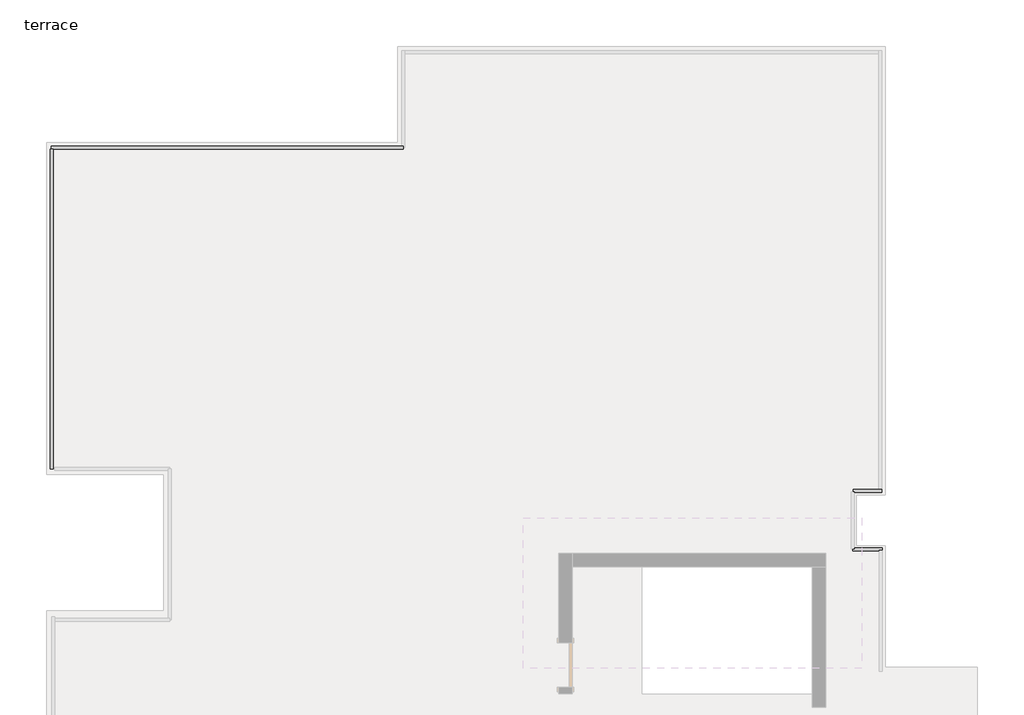
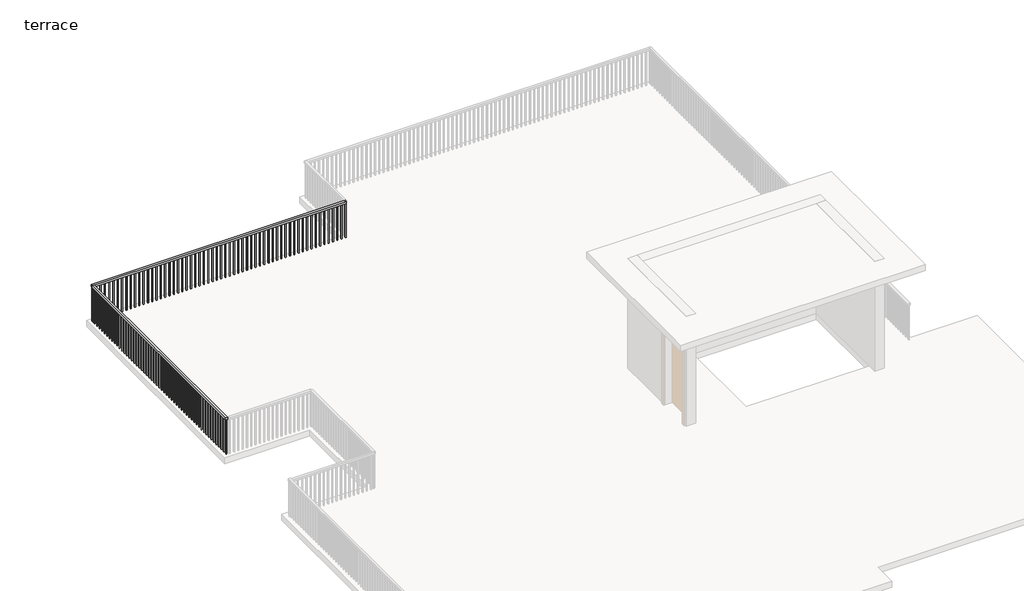
# One storey, part 5 of 7: 4 railings.
"""IFC4 building model written with IfcOpenShell, lengths in millimetres."""

from ifc_helpers import new_model, si_unit, frame, origin, place, context, project, spatial, polyline, outline, extrude, element, save

model = new_model("IFC4")

# Units and contexts
model_context = context("Model", 3, world=origin())
ifc_project = project(units=[si_unit("LENGTHUNIT", "METRE", prefix="MILLI")], contexts=[model_context])

# Site, building, storey
site = spatial("IfcSite", under=ifc_project)
building = spatial("IfcBuilding", under=site)
storey = spatial("IfcBuildingStorey", under=building, Name="terrace", Elevation=3810.0)

# Railings
placement = place(None, origin())
element("IfcRailing", 1, ObjectType="Handrail - Rectangular", at=placement, inside=storey, context=model_context, shape_type="SweptSolid", body=[
    extrude(outline(polyline([(-14404.2890129, 10982.627622), (-14404.2890129, 11033.427622), (-8409.8890129, 11033.427622), (-8409.8890129, 10982.627622), (-14404.2890129, 10982.627622)])), frame((0.0, 0.0, 4673.6), z_axis=(0.0, 0.0, 1.0), x_axis=(1.0, 0.0, 0.0)), (0.0, 0.0, 1.0), 50.8),
    extrude(outline(polyline([(-8521.0140129, 10998.502622), (-8521.0140129, 11017.552622), (-8501.9640129, 11017.552622), (-8501.9640129, 10998.502622), (-8521.0140129, 10998.502622)])), frame((0.0, 0.0, 3810.0), z_axis=(0.0, 0.0, 1.0), x_axis=(1.0, 0.0, 0.0)), (0.0, 0.0, 1.0), 863.6),
    extrude(outline(polyline([(-8622.6140129, 10998.502622), (-8622.6140129, 11017.552622), (-8603.5640129, 11017.552622), (-8603.5640129, 10998.502622), (-8622.6140129, 10998.502622)])), frame((0.0, 0.0, 3810.0), z_axis=(0.0, 0.0, 1.0), x_axis=(1.0, 0.0, 0.0)), (0.0, 0.0, 1.0), 863.6),
    extrude(outline(polyline([(-8724.2140129, 10998.502622), (-8724.2140129, 11017.552622), (-8705.1640129, 11017.552622), (-8705.1640129, 10998.502622), (-8724.2140129, 10998.502622)])), frame((0.0, 0.0, 3810.0), z_axis=(0.0, 0.0, 1.0), x_axis=(1.0, 0.0, 0.0)), (0.0, 0.0, 1.0), 863.6),
    extrude(outline(polyline([(-8825.8140129, 10998.502622), (-8825.8140129, 11017.552622), (-8806.7640129, 11017.552622), (-8806.7640129, 10998.502622), (-8825.8140129, 10998.502622)])), frame((0.0, 0.0, 3810.0), z_axis=(0.0, 0.0, 1.0), x_axis=(1.0, 0.0, 0.0)), (0.0, 0.0, 1.0), 863.6),
    extrude(outline(polyline([(-8927.4140129, 10998.502622), (-8927.4140129, 11017.552622), (-8908.3640129, 11017.552622), (-8908.3640129, 10998.502622), (-8927.4140129, 10998.502622)])), frame((0.0, 0.0, 3810.0), z_axis=(0.0, 0.0, 1.0), x_axis=(1.0, 0.0, 0.0)), (0.0, 0.0, 1.0), 863.6),
    extrude(outline(polyline([(-9029.0140129, 10998.502622), (-9029.0140129, 11017.552622), (-9009.9640129, 11017.552622), (-9009.9640129, 10998.502622), (-9029.0140129, 10998.502622)])), frame((0.0, 0.0, 3810.0), z_axis=(0.0, 0.0, 1.0), x_axis=(1.0, 0.0, 0.0)), (0.0, 0.0, 1.0), 863.6),
    extrude(outline(polyline([(-9130.6140129, 10998.502622), (-9130.6140129, 11017.552622), (-9111.5640129, 11017.552622), (-9111.5640129, 10998.502622), (-9130.6140129, 10998.502622)])), frame((0.0, 0.0, 3810.0), z_axis=(0.0, 0.0, 1.0), x_axis=(1.0, 0.0, 0.0)), (0.0, 0.0, 1.0), 863.6),
    extrude(outline(polyline([(-9232.2140129, 10998.502622), (-9232.2140129, 11017.552622), (-9213.1640129, 11017.552622), (-9213.1640129, 10998.502622), (-9232.2140129, 10998.502622)])), frame((0.0, 0.0, 3810.0), z_axis=(0.0, 0.0, 1.0), x_axis=(1.0, 0.0, 0.0)), (0.0, 0.0, 1.0), 863.6),
    extrude(outline(polyline([(-9333.8140129, 10998.502622), (-9333.8140129, 11017.552622), (-9314.7640129, 11017.552622), (-9314.7640129, 10998.502622), (-9333.8140129, 10998.502622)])), frame((0.0, 0.0, 3810.0), z_axis=(0.0, 0.0, 1.0), x_axis=(1.0, 0.0, 0.0)), (0.0, 0.0, 1.0), 863.6),
    extrude(outline(polyline([(-9435.4140129, 10998.502622), (-9435.4140129, 11017.552622), (-9416.3640129, 11017.552622), (-9416.3640129, 10998.502622), (-9435.4140129, 10998.502622)])), frame((0.0, 0.0, 3810.0), z_axis=(0.0, 0.0, 1.0), x_axis=(1.0, 0.0, 0.0)), (0.0, 0.0, 1.0), 863.6),
    extrude(outline(polyline([(-9537.0140129, 10998.502622), (-9537.0140129, 11017.552622), (-9517.9640129, 11017.552622), (-9517.9640129, 10998.502622), (-9537.0140129, 10998.502622)])), frame((0.0, 0.0, 3810.0), z_axis=(0.0, 0.0, 1.0), x_axis=(1.0, 0.0, 0.0)), (0.0, 0.0, 1.0), 863.6),
    extrude(outline(polyline([(-9638.6140129, 10998.502622), (-9638.6140129, 11017.552622), (-9619.5640129, 11017.552622), (-9619.5640129, 10998.502622), (-9638.6140129, 10998.502622)])), frame((0.0, 0.0, 3810.0), z_axis=(0.0, 0.0, 1.0), x_axis=(1.0, 0.0, 0.0)), (0.0, 0.0, 1.0), 863.6),
    extrude(outline(polyline([(-9740.2140129, 10998.502622), (-9740.2140129, 11017.552622), (-9721.1640129, 11017.552622), (-9721.1640129, 10998.502622), (-9740.2140129, 10998.502622)])), frame((0.0, 0.0, 3810.0), z_axis=(0.0, 0.0, 1.0), x_axis=(1.0, 0.0, 0.0)), (0.0, 0.0, 1.0), 863.6),
    extrude(outline(polyline([(-9841.8140129, 10998.502622), (-9841.8140129, 11017.552622), (-9822.7640129, 11017.552622), (-9822.7640129, 10998.502622), (-9841.8140129, 10998.502622)])), frame((0.0, 0.0, 3810.0), z_axis=(0.0, 0.0, 1.0), x_axis=(1.0, 0.0, 0.0)), (0.0, 0.0, 1.0), 863.6),
    extrude(outline(polyline([(-9943.4140129, 10998.502622), (-9943.4140129, 11017.552622), (-9924.3640129, 11017.552622), (-9924.3640129, 10998.502622), (-9943.4140129, 10998.502622)])), frame((0.0, 0.0, 3810.0), z_axis=(0.0, 0.0, 1.0), x_axis=(1.0, 0.0, 0.0)), (0.0, 0.0, 1.0), 863.6),
    extrude(outline(polyline([(-10045.0140129, 10998.502622), (-10045.0140129, 11017.552622), (-10025.9640129, 11017.552622), (-10025.9640129, 10998.502622), (-10045.0140129, 10998.502622)])), frame((0.0, 0.0, 3810.0), z_axis=(0.0, 0.0, 1.0), x_axis=(1.0, 0.0, 0.0)), (0.0, 0.0, 1.0), 863.6),
    extrude(outline(polyline([(-10146.6140129, 10998.502622), (-10146.6140129, 11017.552622), (-10127.5640129, 11017.552622), (-10127.5640129, 10998.502622), (-10146.6140129, 10998.502622)])), frame((0.0, 0.0, 3810.0), z_axis=(0.0, 0.0, 1.0), x_axis=(1.0, 0.0, 0.0)), (0.0, 0.0, 1.0), 863.6),
    extrude(outline(polyline([(-10248.2140129, 10998.502622), (-10248.2140129, 11017.552622), (-10229.1640129, 11017.552622), (-10229.1640129, 10998.502622), (-10248.2140129, 10998.502622)])), frame((0.0, 0.0, 3810.0), z_axis=(0.0, 0.0, 1.0), x_axis=(1.0, 0.0, 0.0)), (0.0, 0.0, 1.0), 863.6),
    extrude(outline(polyline([(-10349.8140129, 10998.502622), (-10349.8140129, 11017.552622), (-10330.7640129, 11017.552622), (-10330.7640129, 10998.502622), (-10349.8140129, 10998.502622)])), frame((0.0, 0.0, 3810.0), z_axis=(0.0, 0.0, 1.0), x_axis=(1.0, 0.0, 0.0)), (0.0, 0.0, 1.0), 863.6),
    extrude(outline(polyline([(-10451.4140129, 10998.502622), (-10451.4140129, 11017.552622), (-10432.3640129, 11017.552622), (-10432.3640129, 10998.502622), (-10451.4140129, 10998.502622)])), frame((0.0, 0.0, 3810.0), z_axis=(0.0, 0.0, 1.0), x_axis=(1.0, 0.0, 0.0)), (0.0, 0.0, 1.0), 863.6),
    extrude(outline(polyline([(-10553.0140129, 10998.502622), (-10553.0140129, 11017.552622), (-10533.9640129, 11017.552622), (-10533.9640129, 10998.502622), (-10553.0140129, 10998.502622)])), frame((0.0, 0.0, 3810.0), z_axis=(0.0, 0.0, 1.0), x_axis=(1.0, 0.0, 0.0)), (0.0, 0.0, 1.0), 863.6),
    extrude(outline(polyline([(-10654.6140129, 10998.502622), (-10654.6140129, 11017.552622), (-10635.5640129, 11017.552622), (-10635.5640129, 10998.502622), (-10654.6140129, 10998.502622)])), frame((0.0, 0.0, 3810.0), z_axis=(0.0, 0.0, 1.0), x_axis=(1.0, 0.0, 0.0)), (0.0, 0.0, 1.0), 863.6),
    extrude(outline(polyline([(-10756.2140129, 10998.502622), (-10756.2140129, 11017.552622), (-10737.1640129, 11017.552622), (-10737.1640129, 10998.502622), (-10756.2140129, 10998.502622)])), frame((0.0, 0.0, 3810.0), z_axis=(0.0, 0.0, 1.0), x_axis=(1.0, 0.0, 0.0)), (0.0, 0.0, 1.0), 863.6),
    extrude(outline(polyline([(-10857.8140129, 10998.502622), (-10857.8140129, 11017.552622), (-10838.7640129, 11017.552622), (-10838.7640129, 10998.502622), (-10857.8140129, 10998.502622)])), frame((0.0, 0.0, 3810.0), z_axis=(0.0, 0.0, 1.0), x_axis=(1.0, 0.0, 0.0)), (0.0, 0.0, 1.0), 863.6),
    extrude(outline(polyline([(-10959.4140129, 10998.502622), (-10959.4140129, 11017.552622), (-10940.3640129, 11017.552622), (-10940.3640129, 10998.502622), (-10959.4140129, 10998.502622)])), frame((0.0, 0.0, 3810.0), z_axis=(0.0, 0.0, 1.0), x_axis=(1.0, 0.0, 0.0)), (0.0, 0.0, 1.0), 863.6),
    extrude(outline(polyline([(-11061.0140129, 10998.502622), (-11061.0140129, 11017.552622), (-11041.9640129, 11017.552622), (-11041.9640129, 10998.502622), (-11061.0140129, 10998.502622)])), frame((0.0, 0.0, 3810.0), z_axis=(0.0, 0.0, 1.0), x_axis=(1.0, 0.0, 0.0)), (0.0, 0.0, 1.0), 863.6),
    extrude(outline(polyline([(-11162.6140129, 10998.502622), (-11162.6140129, 11017.552622), (-11143.5640129, 11017.552622), (-11143.5640129, 10998.502622), (-11162.6140129, 10998.502622)])), frame((0.0, 0.0, 3810.0), z_axis=(0.0, 0.0, 1.0), x_axis=(1.0, 0.0, 0.0)), (0.0, 0.0, 1.0), 863.6),
    extrude(outline(polyline([(-11264.2140129, 10998.502622), (-11264.2140129, 11017.552622), (-11245.1640129, 11017.552622), (-11245.1640129, 10998.502622), (-11264.2140129, 10998.502622)])), frame((0.0, 0.0, 3810.0), z_axis=(0.0, 0.0, 1.0), x_axis=(1.0, 0.0, 0.0)), (0.0, 0.0, 1.0), 863.6),
    extrude(outline(polyline([(-11365.8140129, 10998.502622), (-11365.8140129, 11017.552622), (-11346.7640129, 11017.552622), (-11346.7640129, 10998.502622), (-11365.8140129, 10998.502622)])), frame((0.0, 0.0, 3810.0), z_axis=(0.0, 0.0, 1.0), x_axis=(1.0, 0.0, 0.0)), (0.0, 0.0, 1.0), 863.6),
    extrude(outline(polyline([(-11467.4140129, 10998.502622), (-11467.4140129, 11017.552622), (-11448.3640129, 11017.552622), (-11448.3640129, 10998.502622), (-11467.4140129, 10998.502622)])), frame((0.0, 0.0, 3810.0), z_axis=(0.0, 0.0, 1.0), x_axis=(1.0, 0.0, 0.0)), (0.0, 0.0, 1.0), 863.6),
    extrude(outline(polyline([(-11569.0140129, 10998.502622), (-11569.0140129, 11017.552622), (-11549.9640129, 11017.552622), (-11549.9640129, 10998.502622), (-11569.0140129, 10998.502622)])), frame((0.0, 0.0, 3810.0), z_axis=(0.0, 0.0, 1.0), x_axis=(1.0, 0.0, 0.0)), (0.0, 0.0, 1.0), 863.6),
    extrude(outline(polyline([(-11670.6140129, 10998.502622), (-11670.6140129, 11017.552622), (-11651.5640129, 11017.552622), (-11651.5640129, 10998.502622), (-11670.6140129, 10998.502622)])), frame((0.0, 0.0, 3810.0), z_axis=(0.0, 0.0, 1.0), x_axis=(1.0, 0.0, 0.0)), (0.0, 0.0, 1.0), 863.6),
    extrude(outline(polyline([(-11772.2140129, 10998.502622), (-11772.2140129, 11017.552622), (-11753.1640129, 11017.552622), (-11753.1640129, 10998.502622), (-11772.2140129, 10998.502622)])), frame((0.0, 0.0, 3810.0), z_axis=(0.0, 0.0, 1.0), x_axis=(1.0, 0.0, 0.0)), (0.0, 0.0, 1.0), 863.6),
    extrude(outline(polyline([(-11873.8140129, 10998.502622), (-11873.8140129, 11017.552622), (-11854.7640129, 11017.552622), (-11854.7640129, 10998.502622), (-11873.8140129, 10998.502622)])), frame((0.0, 0.0, 3810.0), z_axis=(0.0, 0.0, 1.0), x_axis=(1.0, 0.0, 0.0)), (0.0, 0.0, 1.0), 863.6),
    extrude(outline(polyline([(-11975.4140129, 10998.502622), (-11975.4140129, 11017.552622), (-11956.3640129, 11017.552622), (-11956.3640129, 10998.502622), (-11975.4140129, 10998.502622)])), frame((0.0, 0.0, 3810.0), z_axis=(0.0, 0.0, 1.0), x_axis=(1.0, 0.0, 0.0)), (0.0, 0.0, 1.0), 863.6),
    extrude(outline(polyline([(-12077.0140129, 10998.502622), (-12077.0140129, 11017.552622), (-12057.9640129, 11017.552622), (-12057.9640129, 10998.502622), (-12077.0140129, 10998.502622)])), frame((0.0, 0.0, 3810.0), z_axis=(0.0, 0.0, 1.0), x_axis=(1.0, 0.0, 0.0)), (0.0, 0.0, 1.0), 863.6),
    extrude(outline(polyline([(-12178.6140129, 10998.502622), (-12178.6140129, 11017.552622), (-12159.5640129, 11017.552622), (-12159.5640129, 10998.502622), (-12178.6140129, 10998.502622)])), frame((0.0, 0.0, 3810.0), z_axis=(0.0, 0.0, 1.0), x_axis=(1.0, 0.0, 0.0)), (0.0, 0.0, 1.0), 863.6),
    extrude(outline(polyline([(-12280.2140129, 10998.502622), (-12280.2140129, 11017.552622), (-12261.1640129, 11017.552622), (-12261.1640129, 10998.502622), (-12280.2140129, 10998.502622)])), frame((0.0, 0.0, 3810.0), z_axis=(0.0, 0.0, 1.0), x_axis=(1.0, 0.0, 0.0)), (0.0, 0.0, 1.0), 863.6),
    extrude(outline(polyline([(-12381.8140129, 10998.502622), (-12381.8140129, 11017.552622), (-12362.7640129, 11017.552622), (-12362.7640129, 10998.502622), (-12381.8140129, 10998.502622)])), frame((0.0, 0.0, 3810.0), z_axis=(0.0, 0.0, 1.0), x_axis=(1.0, 0.0, 0.0)), (0.0, 0.0, 1.0), 863.6),
    extrude(outline(polyline([(-12483.4140129, 10998.502622), (-12483.4140129, 11017.552622), (-12464.3640129, 11017.552622), (-12464.3640129, 10998.502622), (-12483.4140129, 10998.502622)])), frame((0.0, 0.0, 3810.0), z_axis=(0.0, 0.0, 1.0), x_axis=(1.0, 0.0, 0.0)), (0.0, 0.0, 1.0), 863.6),
    extrude(outline(polyline([(-12585.0140129, 10998.502622), (-12585.0140129, 11017.552622), (-12565.9640129, 11017.552622), (-12565.9640129, 10998.502622), (-12585.0140129, 10998.502622)])), frame((0.0, 0.0, 3810.0), z_axis=(0.0, 0.0, 1.0), x_axis=(1.0, 0.0, 0.0)), (0.0, 0.0, 1.0), 863.6),
    extrude(outline(polyline([(-12686.6140129, 10998.502622), (-12686.6140129, 11017.552622), (-12667.5640129, 11017.552622), (-12667.5640129, 10998.502622), (-12686.6140129, 10998.502622)])), frame((0.0, 0.0, 3810.0), z_axis=(0.0, 0.0, 1.0), x_axis=(1.0, 0.0, 0.0)), (0.0, 0.0, 1.0), 863.6),
    extrude(outline(polyline([(-12788.2140129, 10998.502622), (-12788.2140129, 11017.552622), (-12769.1640129, 11017.552622), (-12769.1640129, 10998.502622), (-12788.2140129, 10998.502622)])), frame((0.0, 0.0, 3810.0), z_axis=(0.0, 0.0, 1.0), x_axis=(1.0, 0.0, 0.0)), (0.0, 0.0, 1.0), 863.6),
    extrude(outline(polyline([(-12889.8140129, 10998.502622), (-12889.8140129, 11017.552622), (-12870.7640129, 11017.552622), (-12870.7640129, 10998.502622), (-12889.8140129, 10998.502622)])), frame((0.0, 0.0, 3810.0), z_axis=(0.0, 0.0, 1.0), x_axis=(1.0, 0.0, 0.0)), (0.0, 0.0, 1.0), 863.6),
    extrude(outline(polyline([(-12991.4140129, 10998.502622), (-12991.4140129, 11017.552622), (-12972.3640129, 11017.552622), (-12972.3640129, 10998.502622), (-12991.4140129, 10998.502622)])), frame((0.0, 0.0, 3810.0), z_axis=(0.0, 0.0, 1.0), x_axis=(1.0, 0.0, 0.0)), (0.0, 0.0, 1.0), 863.6),
    extrude(outline(polyline([(-13093.0140129, 10998.502622), (-13093.0140129, 11017.552622), (-13073.9640129, 11017.552622), (-13073.9640129, 10998.502622), (-13093.0140129, 10998.502622)])), frame((0.0, 0.0, 3810.0), z_axis=(0.0, 0.0, 1.0), x_axis=(1.0, 0.0, 0.0)), (0.0, 0.0, 1.0), 863.6),
    extrude(outline(polyline([(-13194.6140129, 10998.502622), (-13194.6140129, 11017.552622), (-13175.5640129, 11017.552622), (-13175.5640129, 10998.502622), (-13194.6140129, 10998.502622)])), frame((0.0, 0.0, 3810.0), z_axis=(0.0, 0.0, 1.0), x_axis=(1.0, 0.0, 0.0)), (0.0, 0.0, 1.0), 863.6),
    extrude(outline(polyline([(-13296.2140129, 10998.502622), (-13296.2140129, 11017.552622), (-13277.1640129, 11017.552622), (-13277.1640129, 10998.502622), (-13296.2140129, 10998.502622)])), frame((0.0, 0.0, 3810.0), z_axis=(0.0, 0.0, 1.0), x_axis=(1.0, 0.0, 0.0)), (0.0, 0.0, 1.0), 863.6),
    extrude(outline(polyline([(-13397.8140129, 10998.502622), (-13397.8140129, 11017.552622), (-13378.7640129, 11017.552622), (-13378.7640129, 10998.502622), (-13397.8140129, 10998.502622)])), frame((0.0, 0.0, 3810.0), z_axis=(0.0, 0.0, 1.0), x_axis=(1.0, 0.0, 0.0)), (0.0, 0.0, 1.0), 863.6),
    extrude(outline(polyline([(-13499.4140129, 10998.502622), (-13499.4140129, 11017.552622), (-13480.3640129, 11017.552622), (-13480.3640129, 10998.502622), (-13499.4140129, 10998.502622)])), frame((0.0, 0.0, 3810.0), z_axis=(0.0, 0.0, 1.0), x_axis=(1.0, 0.0, 0.0)), (0.0, 0.0, 1.0), 863.6),
    extrude(outline(polyline([(-13601.0140129, 10998.502622), (-13601.0140129, 11017.552622), (-13581.9640129, 11017.552622), (-13581.9640129, 10998.502622), (-13601.0140129, 10998.502622)])), frame((0.0, 0.0, 3810.0), z_axis=(0.0, 0.0, 1.0), x_axis=(1.0, 0.0, 0.0)), (0.0, 0.0, 1.0), 863.6),
    extrude(outline(polyline([(-13702.6140129, 10998.502622), (-13702.6140129, 11017.552622), (-13683.5640129, 11017.552622), (-13683.5640129, 10998.502622), (-13702.6140129, 10998.502622)])), frame((0.0, 0.0, 3810.0), z_axis=(0.0, 0.0, 1.0), x_axis=(1.0, 0.0, 0.0)), (0.0, 0.0, 1.0), 863.6),
    extrude(outline(polyline([(-13804.2140129, 10998.502622), (-13804.2140129, 11017.552622), (-13785.1640129, 11017.552622), (-13785.1640129, 10998.502622), (-13804.2140129, 10998.502622)])), frame((0.0, 0.0, 3810.0), z_axis=(0.0, 0.0, 1.0), x_axis=(1.0, 0.0, 0.0)), (0.0, 0.0, 1.0), 863.6),
    extrude(outline(polyline([(-13905.8140129, 10998.502622), (-13905.8140129, 11017.552622), (-13886.7640129, 11017.552622), (-13886.7640129, 10998.502622), (-13905.8140129, 10998.502622)])), frame((0.0, 0.0, 3810.0), z_axis=(0.0, 0.0, 1.0), x_axis=(1.0, 0.0, 0.0)), (0.0, 0.0, 1.0), 863.6),
    extrude(outline(polyline([(-14007.4140129, 10998.502622), (-14007.4140129, 11017.552622), (-13988.3640129, 11017.552622), (-13988.3640129, 10998.502622), (-14007.4140129, 10998.502622)])), frame((0.0, 0.0, 3810.0), z_axis=(0.0, 0.0, 1.0), x_axis=(1.0, 0.0, 0.0)), (0.0, 0.0, 1.0), 863.6),
    extrude(outline(polyline([(-14109.0140129, 10998.502622), (-14109.0140129, 11017.552622), (-14089.9640129, 11017.552622), (-14089.9640129, 10998.502622), (-14109.0140129, 10998.502622)])), frame((0.0, 0.0, 3810.0), z_axis=(0.0, 0.0, 1.0), x_axis=(1.0, 0.0, 0.0)), (0.0, 0.0, 1.0), 863.6),
    extrude(outline(polyline([(-14210.6140129, 10998.502622), (-14210.6140129, 11017.552622), (-14191.5640129, 11017.552622), (-14191.5640129, 10998.502622), (-14210.6140129, 10998.502622)])), frame((0.0, 0.0, 3810.0), z_axis=(0.0, 0.0, 1.0), x_axis=(1.0, 0.0, 0.0)), (0.0, 0.0, 1.0), 863.6),
    extrude(outline(polyline([(-14312.2140129, 10998.502622), (-14312.2140129, 11017.552622), (-14293.1640129, 11017.552622), (-14293.1640129, 10998.502622), (-14312.2140129, 10998.502622)])), frame((0.0, 0.0, 3810.0), z_axis=(0.0, 0.0, 1.0), x_axis=(1.0, 0.0, 0.0)), (0.0, 0.0, 1.0), 863.6),
    extrude(outline(polyline([(-8428.9390129, 10998.502622), (-8428.9390129, 11017.552622), (-8409.8890129, 11017.552622), (-8409.8890129, 10998.502622), (-8428.9390129, 10998.502622)])), frame((0.0, 0.0, 3810.0), z_axis=(0.0, 0.0, 1.0), x_axis=(1.0, 0.0, 0.0)), (0.0, 0.0, 1.0), 863.6),
    extrude(outline(polyline([(-14404.2890129, 10998.502622), (-14404.2890129, 11017.552622), (-14385.2390129, 11017.552622), (-14385.2390129, 10998.502622), (-14404.2890129, 10998.502622)])), frame((0.0, 0.0, 3810.0), z_axis=(0.0, 0.0, 1.0), x_axis=(1.0, 0.0, 0.0)), (0.0, 0.0, 1.0), 863.6),
])
element("IfcRailing", 2, ObjectType="Handrail - Rectangular", at=placement, inside=storey, context=model_context, shape_type="SweptSolid", body=[
    extrude(outline(polyline([(-256.4890129, 5178.727622), (-256.4890129, 5127.927622), (-739.0890129, 5127.927622), (-739.0890129, 5178.727622), (-256.4890129, 5178.727622)])), frame((0.0, 0.0, 4673.6), z_axis=(0.0, 0.0, 1.0), x_axis=(1.0, 0.0, 0.0)), (0.0, 0.0, 1.0), 50.8),
    extrude(outline(polyline([(-653.3640129, 5162.852622), (-653.3640129, 5143.802622), (-672.4140129, 5143.802622), (-672.4140129, 5162.852622), (-653.3640129, 5162.852622)])), frame((0.0, 0.0, 3810.0), z_axis=(0.0, 0.0, 1.0), x_axis=(1.0, 0.0, 0.0)), (0.0, 0.0, 1.0), 863.6),
    extrude(outline(polyline([(-551.7640129, 5162.852622), (-551.7640129, 5143.802622), (-570.8140129, 5143.802622), (-570.8140129, 5162.852622), (-551.7640129, 5162.852622)])), frame((0.0, 0.0, 3810.0), z_axis=(0.0, 0.0, 1.0), x_axis=(1.0, 0.0, 0.0)), (0.0, 0.0, 1.0), 863.6),
    extrude(outline(polyline([(-450.1640129, 5162.852622), (-450.1640129, 5143.802622), (-469.2140129, 5143.802622), (-469.2140129, 5162.852622), (-450.1640129, 5162.852622)])), frame((0.0, 0.0, 3810.0), z_axis=(0.0, 0.0, 1.0), x_axis=(1.0, 0.0, 0.0)), (0.0, 0.0, 1.0), 863.6),
    extrude(outline(polyline([(-348.5640129, 5162.852622), (-348.5640129, 5143.802622), (-367.6140129, 5143.802622), (-367.6140129, 5162.852622), (-348.5640129, 5162.852622)])), frame((0.0, 0.0, 3810.0), z_axis=(0.0, 0.0, 1.0), x_axis=(1.0, 0.0, 0.0)), (0.0, 0.0, 1.0), 863.6),
    extrude(outline(polyline([(-720.0390129, 5162.852622), (-720.0390129, 5143.802622), (-739.0890129, 5143.802622), (-739.0890129, 5162.852622), (-720.0390129, 5162.852622)])), frame((0.0, 0.0, 3810.0), z_axis=(0.0, 0.0, 1.0), x_axis=(1.0, 0.0, 0.0)), (0.0, 0.0, 1.0), 863.6),
    extrude(outline(polyline([(-256.4890129, 5162.852622), (-256.4890129, 5143.802622), (-275.5390129, 5143.802622), (-275.5390129, 5162.852622), (-256.4890129, 5162.852622)])), frame((0.0, 0.0, 3810.0), z_axis=(0.0, 0.0, 1.0), x_axis=(1.0, 0.0, 0.0)), (0.0, 0.0, 1.0), 863.6),
])
element("IfcRailing", 3, ObjectType="Handrail - Rectangular", at=placement, inside=storey, context=model_context, shape_type="SweptSolid", body=[
    extrude(outline(polyline([(-751.7890129, 4130.977622), (-751.7890129, 4181.777622), (-243.7890129, 4181.777622), (-243.7890129, 4130.977622), (-751.7890129, 4130.977622)])), frame((0.0, 0.0, 4673.6), z_axis=(0.0, 0.0, 1.0), x_axis=(1.0, 0.0, 0.0)), (0.0, 0.0, 1.0), 50.8),
    extrude(outline(polyline([(-354.9140129, 4146.852622), (-354.9140129, 4165.902622), (-335.8640129, 4165.902622), (-335.8640129, 4146.852622), (-354.9140129, 4146.852622)])), frame((0.0, 0.0, 3810.0), z_axis=(0.0, 0.0, 1.0), x_axis=(1.0, 0.0, 0.0)), (0.0, 0.0, 1.0), 863.6),
    extrude(outline(polyline([(-456.5140129, 4146.852622), (-456.5140129, 4165.902622), (-437.4640129, 4165.902622), (-437.4640129, 4146.852622), (-456.5140129, 4146.852622)])), frame((0.0, 0.0, 3810.0), z_axis=(0.0, 0.0, 1.0), x_axis=(1.0, 0.0, 0.0)), (0.0, 0.0, 1.0), 863.6),
    extrude(outline(polyline([(-558.1140129, 4146.852622), (-558.1140129, 4165.902622), (-539.0640129, 4165.902622), (-539.0640129, 4146.852622), (-558.1140129, 4146.852622)])), frame((0.0, 0.0, 3810.0), z_axis=(0.0, 0.0, 1.0), x_axis=(1.0, 0.0, 0.0)), (0.0, 0.0, 1.0), 863.6),
    extrude(outline(polyline([(-659.7140129, 4146.852622), (-659.7140129, 4165.902622), (-640.6640129, 4165.902622), (-640.6640129, 4146.852622), (-659.7140129, 4146.852622)])), frame((0.0, 0.0, 3810.0), z_axis=(0.0, 0.0, 1.0), x_axis=(1.0, 0.0, 0.0)), (0.0, 0.0, 1.0), 863.6),
    extrude(outline(polyline([(-262.8390129, 4146.852622), (-262.8390129, 4165.902622), (-243.7890129, 4165.902622), (-243.7890129, 4146.852622), (-262.8390129, 4146.852622)])), frame((0.0, 0.0, 3810.0), z_axis=(0.0, 0.0, 1.0), x_axis=(1.0, 0.0, 0.0)), (0.0, 0.0, 1.0), 863.6),
    extrude(outline(polyline([(-751.7890129, 4146.852622), (-751.7890129, 4165.902622), (-732.7390129, 4165.902622), (-732.7390129, 4146.852622), (-751.7890129, 4146.852622)])), frame((0.0, 0.0, 3810.0), z_axis=(0.0, 0.0, 1.0), x_axis=(1.0, 0.0, 0.0)), (0.0, 0.0, 1.0), 863.6),
])
element("IfcRailing", 4, ObjectType="Handrail - Rectangular", at=placement, inside=storey, context=model_context, shape_type="SweptSolid", body=[
    extrude(outline(polyline([(-14366.1890129, 5527.977622), (-14416.9890129, 5527.977622), (-14416.9890129, 10982.627622), (-14366.1890129, 10982.627622), (-14366.1890129, 5527.977622)])), frame((0.0, 0.0, 4673.6), z_axis=(0.0, 0.0, 1.0), x_axis=(1.0, 0.0, 0.0)), (0.0, 0.0, 1.0), 50.8),
    extrude(outline(polyline([(-14382.0640129, 10903.252622), (-14401.1140129, 10903.252622), (-14401.1140129, 10922.302622), (-14382.0640129, 10922.302622), (-14382.0640129, 10903.252622)])), frame((0.0, 0.0, 3810.0), z_axis=(0.0, 0.0, 1.0), x_axis=(1.0, 0.0, 0.0)), (0.0, 0.0, 1.0), 863.6),
    extrude(outline(polyline([(-14382.0640129, 10801.652622), (-14401.1140129, 10801.652622), (-14401.1140129, 10820.702622), (-14382.0640129, 10820.702622), (-14382.0640129, 10801.652622)])), frame((0.0, 0.0, 3810.0), z_axis=(0.0, 0.0, 1.0), x_axis=(1.0, 0.0, 0.0)), (0.0, 0.0, 1.0), 863.6),
    extrude(outline(polyline([(-14382.0640129, 10700.052622), (-14401.1140129, 10700.052622), (-14401.1140129, 10719.102622), (-14382.0640129, 10719.102622), (-14382.0640129, 10700.052622)])), frame((0.0, 0.0, 3810.0), z_axis=(0.0, 0.0, 1.0), x_axis=(1.0, 0.0, 0.0)), (0.0, 0.0, 1.0), 863.6),
    extrude(outline(polyline([(-14382.0640129, 10598.452622), (-14401.1140129, 10598.452622), (-14401.1140129, 10617.502622), (-14382.0640129, 10617.502622), (-14382.0640129, 10598.452622)])), frame((0.0, 0.0, 3810.0), z_axis=(0.0, 0.0, 1.0), x_axis=(1.0, 0.0, 0.0)), (0.0, 0.0, 1.0), 863.6),
    extrude(outline(polyline([(-14382.0640129, 10496.852622), (-14401.1140129, 10496.852622), (-14401.1140129, 10515.902622), (-14382.0640129, 10515.902622), (-14382.0640129, 10496.852622)])), frame((0.0, 0.0, 3810.0), z_axis=(0.0, 0.0, 1.0), x_axis=(1.0, 0.0, 0.0)), (0.0, 0.0, 1.0), 863.6),
    extrude(outline(polyline([(-14382.0640129, 10395.252622), (-14401.1140129, 10395.252622), (-14401.1140129, 10414.302622), (-14382.0640129, 10414.302622), (-14382.0640129, 10395.252622)])), frame((0.0, 0.0, 3810.0), z_axis=(0.0, 0.0, 1.0), x_axis=(1.0, 0.0, 0.0)), (0.0, 0.0, 1.0), 863.6),
    extrude(outline(polyline([(-14382.0640129, 10293.652622), (-14401.1140129, 10293.652622), (-14401.1140129, 10312.702622), (-14382.0640129, 10312.702622), (-14382.0640129, 10293.652622)])), frame((0.0, 0.0, 3810.0), z_axis=(0.0, 0.0, 1.0), x_axis=(1.0, 0.0, 0.0)), (0.0, 0.0, 1.0), 863.6),
    extrude(outline(polyline([(-14382.0640129, 10192.052622), (-14401.1140129, 10192.052622), (-14401.1140129, 10211.102622), (-14382.0640129, 10211.102622), (-14382.0640129, 10192.052622)])), frame((0.0, 0.0, 3810.0), z_axis=(0.0, 0.0, 1.0), x_axis=(1.0, 0.0, 0.0)), (0.0, 0.0, 1.0), 863.6),
    extrude(outline(polyline([(-14382.0640129, 10090.452622), (-14401.1140129, 10090.452622), (-14401.1140129, 10109.502622), (-14382.0640129, 10109.502622), (-14382.0640129, 10090.452622)])), frame((0.0, 0.0, 3810.0), z_axis=(0.0, 0.0, 1.0), x_axis=(1.0, 0.0, 0.0)), (0.0, 0.0, 1.0), 863.6),
    extrude(outline(polyline([(-14382.0640129, 9988.852622), (-14401.1140129, 9988.852622), (-14401.1140129, 10007.902622), (-14382.0640129, 10007.902622), (-14382.0640129, 9988.852622)])), frame((0.0, 0.0, 3810.0), z_axis=(0.0, 0.0, 1.0), x_axis=(1.0, 0.0, 0.0)), (0.0, 0.0, 1.0), 863.6),
    extrude(outline(polyline([(-14382.0640129, 9887.252622), (-14401.1140129, 9887.252622), (-14401.1140129, 9906.302622), (-14382.0640129, 9906.302622), (-14382.0640129, 9887.252622)])), frame((0.0, 0.0, 3810.0), z_axis=(0.0, 0.0, 1.0), x_axis=(1.0, 0.0, 0.0)), (0.0, 0.0, 1.0), 863.6),
    extrude(outline(polyline([(-14382.0640129, 9785.652622), (-14401.1140129, 9785.652622), (-14401.1140129, 9804.702622), (-14382.0640129, 9804.702622), (-14382.0640129, 9785.652622)])), frame((0.0, 0.0, 3810.0), z_axis=(0.0, 0.0, 1.0), x_axis=(1.0, 0.0, 0.0)), (0.0, 0.0, 1.0), 863.6),
    extrude(outline(polyline([(-14382.0640129, 9684.052622), (-14401.1140129, 9684.052622), (-14401.1140129, 9703.102622), (-14382.0640129, 9703.102622), (-14382.0640129, 9684.052622)])), frame((0.0, 0.0, 3810.0), z_axis=(0.0, 0.0, 1.0), x_axis=(1.0, 0.0, 0.0)), (0.0, 0.0, 1.0), 863.6),
    extrude(outline(polyline([(-14382.0640129, 9582.452622), (-14401.1140129, 9582.452622), (-14401.1140129, 9601.502622), (-14382.0640129, 9601.502622), (-14382.0640129, 9582.452622)])), frame((0.0, 0.0, 3810.0), z_axis=(0.0, 0.0, 1.0), x_axis=(1.0, 0.0, 0.0)), (0.0, 0.0, 1.0), 863.6),
    extrude(outline(polyline([(-14382.0640129, 9480.852622), (-14401.1140129, 9480.852622), (-14401.1140129, 9499.902622), (-14382.0640129, 9499.902622), (-14382.0640129, 9480.852622)])), frame((0.0, 0.0, 3810.0), z_axis=(0.0, 0.0, 1.0), x_axis=(1.0, 0.0, 0.0)), (0.0, 0.0, 1.0), 863.6),
    extrude(outline(polyline([(-14382.0640129, 9379.252622), (-14401.1140129, 9379.252622), (-14401.1140129, 9398.302622), (-14382.0640129, 9398.302622), (-14382.0640129, 9379.252622)])), frame((0.0, 0.0, 3810.0), z_axis=(0.0, 0.0, 1.0), x_axis=(1.0, 0.0, 0.0)), (0.0, 0.0, 1.0), 863.6),
    extrude(outline(polyline([(-14382.0640129, 9277.652622), (-14401.1140129, 9277.652622), (-14401.1140129, 9296.702622), (-14382.0640129, 9296.702622), (-14382.0640129, 9277.652622)])), frame((0.0, 0.0, 3810.0), z_axis=(0.0, 0.0, 1.0), x_axis=(1.0, 0.0, 0.0)), (0.0, 0.0, 1.0), 863.6),
    extrude(outline(polyline([(-14382.0640129, 9176.052622), (-14401.1140129, 9176.052622), (-14401.1140129, 9195.102622), (-14382.0640129, 9195.102622), (-14382.0640129, 9176.052622)])), frame((0.0, 0.0, 3810.0), z_axis=(0.0, 0.0, 1.0), x_axis=(1.0, 0.0, 0.0)), (0.0, 0.0, 1.0), 863.6),
    extrude(outline(polyline([(-14382.0640129, 9074.452622), (-14401.1140129, 9074.452622), (-14401.1140129, 9093.502622), (-14382.0640129, 9093.502622), (-14382.0640129, 9074.452622)])), frame((0.0, 0.0, 3810.0), z_axis=(0.0, 0.0, 1.0), x_axis=(1.0, 0.0, 0.0)), (0.0, 0.0, 1.0), 863.6),
    extrude(outline(polyline([(-14382.0640129, 8972.852622), (-14401.1140129, 8972.852622), (-14401.1140129, 8991.902622), (-14382.0640129, 8991.902622), (-14382.0640129, 8972.852622)])), frame((0.0, 0.0, 3810.0), z_axis=(0.0, 0.0, 1.0), x_axis=(1.0, 0.0, 0.0)), (0.0, 0.0, 1.0), 863.6),
    extrude(outline(polyline([(-14382.0640129, 8871.252622), (-14401.1140129, 8871.252622), (-14401.1140129, 8890.302622), (-14382.0640129, 8890.302622), (-14382.0640129, 8871.252622)])), frame((0.0, 0.0, 3810.0), z_axis=(0.0, 0.0, 1.0), x_axis=(1.0, 0.0, 0.0)), (0.0, 0.0, 1.0), 863.6),
    extrude(outline(polyline([(-14382.0640129, 8769.652622), (-14401.1140129, 8769.652622), (-14401.1140129, 8788.702622), (-14382.0640129, 8788.702622), (-14382.0640129, 8769.652622)])), frame((0.0, 0.0, 3810.0), z_axis=(0.0, 0.0, 1.0), x_axis=(1.0, 0.0, 0.0)), (0.0, 0.0, 1.0), 863.6),
    extrude(outline(polyline([(-14382.0640129, 8668.052622), (-14401.1140129, 8668.052622), (-14401.1140129, 8687.102622), (-14382.0640129, 8687.102622), (-14382.0640129, 8668.052622)])), frame((0.0, 0.0, 3810.0), z_axis=(0.0, 0.0, 1.0), x_axis=(1.0, 0.0, 0.0)), (0.0, 0.0, 1.0), 863.6),
    extrude(outline(polyline([(-14382.0640129, 8566.452622), (-14401.1140129, 8566.452622), (-14401.1140129, 8585.502622), (-14382.0640129, 8585.502622), (-14382.0640129, 8566.452622)])), frame((0.0, 0.0, 3810.0), z_axis=(0.0, 0.0, 1.0), x_axis=(1.0, 0.0, 0.0)), (0.0, 0.0, 1.0), 863.6),
    extrude(outline(polyline([(-14382.0640129, 8464.852622), (-14401.1140129, 8464.852622), (-14401.1140129, 8483.902622), (-14382.0640129, 8483.902622), (-14382.0640129, 8464.852622)])), frame((0.0, 0.0, 3810.0), z_axis=(0.0, 0.0, 1.0), x_axis=(1.0, 0.0, 0.0)), (0.0, 0.0, 1.0), 863.6),
    extrude(outline(polyline([(-14382.0640129, 8363.252622), (-14401.1140129, 8363.252622), (-14401.1140129, 8382.302622), (-14382.0640129, 8382.302622), (-14382.0640129, 8363.252622)])), frame((0.0, 0.0, 3810.0), z_axis=(0.0, 0.0, 1.0), x_axis=(1.0, 0.0, 0.0)), (0.0, 0.0, 1.0), 863.6),
    extrude(outline(polyline([(-14382.0640129, 8261.652622), (-14401.1140129, 8261.652622), (-14401.1140129, 8280.702622), (-14382.0640129, 8280.702622), (-14382.0640129, 8261.652622)])), frame((0.0, 0.0, 3810.0), z_axis=(0.0, 0.0, 1.0), x_axis=(1.0, 0.0, 0.0)), (0.0, 0.0, 1.0), 863.6),
    extrude(outline(polyline([(-14382.0640129, 8160.052622), (-14401.1140129, 8160.052622), (-14401.1140129, 8179.102622), (-14382.0640129, 8179.102622), (-14382.0640129, 8160.052622)])), frame((0.0, 0.0, 3810.0), z_axis=(0.0, 0.0, 1.0), x_axis=(1.0, 0.0, 0.0)), (0.0, 0.0, 1.0), 863.6),
    extrude(outline(polyline([(-14382.0640129, 8058.452622), (-14401.1140129, 8058.452622), (-14401.1140129, 8077.502622), (-14382.0640129, 8077.502622), (-14382.0640129, 8058.452622)])), frame((0.0, 0.0, 3810.0), z_axis=(0.0, 0.0, 1.0), x_axis=(1.0, 0.0, 0.0)), (0.0, 0.0, 1.0), 863.6),
    extrude(outline(polyline([(-14382.0640129, 7956.852622), (-14401.1140129, 7956.852622), (-14401.1140129, 7975.902622), (-14382.0640129, 7975.902622), (-14382.0640129, 7956.852622)])), frame((0.0, 0.0, 3810.0), z_axis=(0.0, 0.0, 1.0), x_axis=(1.0, 0.0, 0.0)), (0.0, 0.0, 1.0), 863.6),
    extrude(outline(polyline([(-14382.0640129, 7855.252622), (-14401.1140129, 7855.252622), (-14401.1140129, 7874.302622), (-14382.0640129, 7874.302622), (-14382.0640129, 7855.252622)])), frame((0.0, 0.0, 3810.0), z_axis=(0.0, 0.0, 1.0), x_axis=(1.0, 0.0, 0.0)), (0.0, 0.0, 1.0), 863.6),
    extrude(outline(polyline([(-14382.0640129, 7753.652622), (-14401.1140129, 7753.652622), (-14401.1140129, 7772.702622), (-14382.0640129, 7772.702622), (-14382.0640129, 7753.652622)])), frame((0.0, 0.0, 3810.0), z_axis=(0.0, 0.0, 1.0), x_axis=(1.0, 0.0, 0.0)), (0.0, 0.0, 1.0), 863.6),
    extrude(outline(polyline([(-14382.0640129, 7652.052622), (-14401.1140129, 7652.052622), (-14401.1140129, 7671.102622), (-14382.0640129, 7671.102622), (-14382.0640129, 7652.052622)])), frame((0.0, 0.0, 3810.0), z_axis=(0.0, 0.0, 1.0), x_axis=(1.0, 0.0, 0.0)), (0.0, 0.0, 1.0), 863.6),
    extrude(outline(polyline([(-14382.0640129, 7550.452622), (-14401.1140129, 7550.452622), (-14401.1140129, 7569.502622), (-14382.0640129, 7569.502622), (-14382.0640129, 7550.452622)])), frame((0.0, 0.0, 3810.0), z_axis=(0.0, 0.0, 1.0), x_axis=(1.0, 0.0, 0.0)), (0.0, 0.0, 1.0), 863.6),
    extrude(outline(polyline([(-14382.0640129, 7448.852622), (-14401.1140129, 7448.852622), (-14401.1140129, 7467.902622), (-14382.0640129, 7467.902622), (-14382.0640129, 7448.852622)])), frame((0.0, 0.0, 3810.0), z_axis=(0.0, 0.0, 1.0), x_axis=(1.0, 0.0, 0.0)), (0.0, 0.0, 1.0), 863.6),
    extrude(outline(polyline([(-14382.0640129, 7347.252622), (-14401.1140129, 7347.252622), (-14401.1140129, 7366.302622), (-14382.0640129, 7366.302622), (-14382.0640129, 7347.252622)])), frame((0.0, 0.0, 3810.0), z_axis=(0.0, 0.0, 1.0), x_axis=(1.0, 0.0, 0.0)), (0.0, 0.0, 1.0), 863.6),
    extrude(outline(polyline([(-14382.0640129, 7245.652622), (-14401.1140129, 7245.652622), (-14401.1140129, 7264.702622), (-14382.0640129, 7264.702622), (-14382.0640129, 7245.652622)])), frame((0.0, 0.0, 3810.0), z_axis=(0.0, 0.0, 1.0), x_axis=(1.0, 0.0, 0.0)), (0.0, 0.0, 1.0), 863.6),
    extrude(outline(polyline([(-14382.0640129, 7144.052622), (-14401.1140129, 7144.052622), (-14401.1140129, 7163.102622), (-14382.0640129, 7163.102622), (-14382.0640129, 7144.052622)])), frame((0.0, 0.0, 3810.0), z_axis=(0.0, 0.0, 1.0), x_axis=(1.0, 0.0, 0.0)), (0.0, 0.0, 1.0), 863.6),
    extrude(outline(polyline([(-14382.0640129, 7042.452622), (-14401.1140129, 7042.452622), (-14401.1140129, 7061.502622), (-14382.0640129, 7061.502622), (-14382.0640129, 7042.452622)])), frame((0.0, 0.0, 3810.0), z_axis=(0.0, 0.0, 1.0), x_axis=(1.0, 0.0, 0.0)), (0.0, 0.0, 1.0), 863.6),
    extrude(outline(polyline([(-14382.0640129, 6940.852622), (-14401.1140129, 6940.852622), (-14401.1140129, 6959.902622), (-14382.0640129, 6959.902622), (-14382.0640129, 6940.852622)])), frame((0.0, 0.0, 3810.0), z_axis=(0.0, 0.0, 1.0), x_axis=(1.0, 0.0, 0.0)), (0.0, 0.0, 1.0), 863.6),
    extrude(outline(polyline([(-14382.0640129, 6839.252622), (-14401.1140129, 6839.252622), (-14401.1140129, 6858.302622), (-14382.0640129, 6858.302622), (-14382.0640129, 6839.252622)])), frame((0.0, 0.0, 3810.0), z_axis=(0.0, 0.0, 1.0), x_axis=(1.0, 0.0, 0.0)), (0.0, 0.0, 1.0), 863.6),
    extrude(outline(polyline([(-14382.0640129, 6737.652622), (-14401.1140129, 6737.652622), (-14401.1140129, 6756.702622), (-14382.0640129, 6756.702622), (-14382.0640129, 6737.652622)])), frame((0.0, 0.0, 3810.0), z_axis=(0.0, 0.0, 1.0), x_axis=(1.0, 0.0, 0.0)), (0.0, 0.0, 1.0), 863.6),
    extrude(outline(polyline([(-14382.0640129, 6636.052622), (-14401.1140129, 6636.052622), (-14401.1140129, 6655.102622), (-14382.0640129, 6655.102622), (-14382.0640129, 6636.052622)])), frame((0.0, 0.0, 3810.0), z_axis=(0.0, 0.0, 1.0), x_axis=(1.0, 0.0, 0.0)), (0.0, 0.0, 1.0), 863.6),
    extrude(outline(polyline([(-14382.0640129, 6534.452622), (-14401.1140129, 6534.452622), (-14401.1140129, 6553.502622), (-14382.0640129, 6553.502622), (-14382.0640129, 6534.452622)])), frame((0.0, 0.0, 3810.0), z_axis=(0.0, 0.0, 1.0), x_axis=(1.0, 0.0, 0.0)), (0.0, 0.0, 1.0), 863.6),
    extrude(outline(polyline([(-14382.0640129, 6432.852622), (-14401.1140129, 6432.852622), (-14401.1140129, 6451.902622), (-14382.0640129, 6451.902622), (-14382.0640129, 6432.852622)])), frame((0.0, 0.0, 3810.0), z_axis=(0.0, 0.0, 1.0), x_axis=(1.0, 0.0, 0.0)), (0.0, 0.0, 1.0), 863.6),
    extrude(outline(polyline([(-14382.0640129, 6331.252622), (-14401.1140129, 6331.252622), (-14401.1140129, 6350.302622), (-14382.0640129, 6350.302622), (-14382.0640129, 6331.252622)])), frame((0.0, 0.0, 3810.0), z_axis=(0.0, 0.0, 1.0), x_axis=(1.0, 0.0, 0.0)), (0.0, 0.0, 1.0), 863.6),
    extrude(outline(polyline([(-14382.0640129, 6229.652622), (-14401.1140129, 6229.652622), (-14401.1140129, 6248.702622), (-14382.0640129, 6248.702622), (-14382.0640129, 6229.652622)])), frame((0.0, 0.0, 3810.0), z_axis=(0.0, 0.0, 1.0), x_axis=(1.0, 0.0, 0.0)), (0.0, 0.0, 1.0), 863.6),
    extrude(outline(polyline([(-14382.0640129, 6128.052622), (-14401.1140129, 6128.052622), (-14401.1140129, 6147.102622), (-14382.0640129, 6147.102622), (-14382.0640129, 6128.052622)])), frame((0.0, 0.0, 3810.0), z_axis=(0.0, 0.0, 1.0), x_axis=(1.0, 0.0, 0.0)), (0.0, 0.0, 1.0), 863.6),
    extrude(outline(polyline([(-14382.0640129, 6026.452622), (-14401.1140129, 6026.452622), (-14401.1140129, 6045.502622), (-14382.0640129, 6045.502622), (-14382.0640129, 6026.452622)])), frame((0.0, 0.0, 3810.0), z_axis=(0.0, 0.0, 1.0), x_axis=(1.0, 0.0, 0.0)), (0.0, 0.0, 1.0), 863.6),
    extrude(outline(polyline([(-14382.0640129, 5924.852622), (-14401.1140129, 5924.852622), (-14401.1140129, 5943.902622), (-14382.0640129, 5943.902622), (-14382.0640129, 5924.852622)])), frame((0.0, 0.0, 3810.0), z_axis=(0.0, 0.0, 1.0), x_axis=(1.0, 0.0, 0.0)), (0.0, 0.0, 1.0), 863.6),
    extrude(outline(polyline([(-14382.0640129, 5823.252622), (-14401.1140129, 5823.252622), (-14401.1140129, 5842.302622), (-14382.0640129, 5842.302622), (-14382.0640129, 5823.252622)])), frame((0.0, 0.0, 3810.0), z_axis=(0.0, 0.0, 1.0), x_axis=(1.0, 0.0, 0.0)), (0.0, 0.0, 1.0), 863.6),
    extrude(outline(polyline([(-14382.0640129, 5721.652622), (-14401.1140129, 5721.652622), (-14401.1140129, 5740.702622), (-14382.0640129, 5740.702622), (-14382.0640129, 5721.652622)])), frame((0.0, 0.0, 3810.0), z_axis=(0.0, 0.0, 1.0), x_axis=(1.0, 0.0, 0.0)), (0.0, 0.0, 1.0), 863.6),
    extrude(outline(polyline([(-14382.0640129, 5620.052622), (-14401.1140129, 5620.052622), (-14401.1140129, 5639.102622), (-14382.0640129, 5639.102622), (-14382.0640129, 5620.052622)])), frame((0.0, 0.0, 3810.0), z_axis=(0.0, 0.0, 1.0), x_axis=(1.0, 0.0, 0.0)), (0.0, 0.0, 1.0), 863.6),
    extrude(outline(polyline([(-14382.0640129, 10963.577622), (-14401.1140129, 10963.577622), (-14401.1140129, 10982.627622), (-14382.0640129, 10982.627622), (-14382.0640129, 10963.577622)])), frame((0.0, 0.0, 3810.0), z_axis=(0.0, 0.0, 1.0), x_axis=(1.0, 0.0, 0.0)), (0.0, 0.0, 1.0), 863.6),
    extrude(outline(polyline([(-14382.0640129, 5527.977622), (-14401.1140129, 5527.977622), (-14401.1140129, 5547.027622), (-14382.0640129, 5547.027622), (-14382.0640129, 5527.977622)])), frame((0.0, 0.0, 3810.0), z_axis=(0.0, 0.0, 1.0), x_axis=(1.0, 0.0, 0.0)), (0.0, 0.0, 1.0), 863.6),
])

save(model, "model.ifc")

# Revit data of these elements
# Type "Handrail - Rectangular"
#   Assembly Code = "C2010400"
#   built-in parameter 1008612 = 0.0416667 (stored number, unit not read)
#   built-in parameter 1008611 = 0.0416667 (stored number, unit not read)
#   built-in parameter 1008609 = 0.333333 (stored number, unit not read)
#   built-in parameter 1008604 = 0.166667 (stored number, unit not read)
#   built-in parameter 1008603 = 0.166667 (stored number, unit not read)
#   Railing Height = 3' - 0"
#   built-in parameter 1008630 = 2
#   built-in parameter 1008610 = 2
#   built-in parameter 1008618 = Baluster - Square : 3/4"
# Elements 1, 2, 3, 4 (IfcRailing, "Handrail - Rectangular")
#   Phase Created = New Construction
